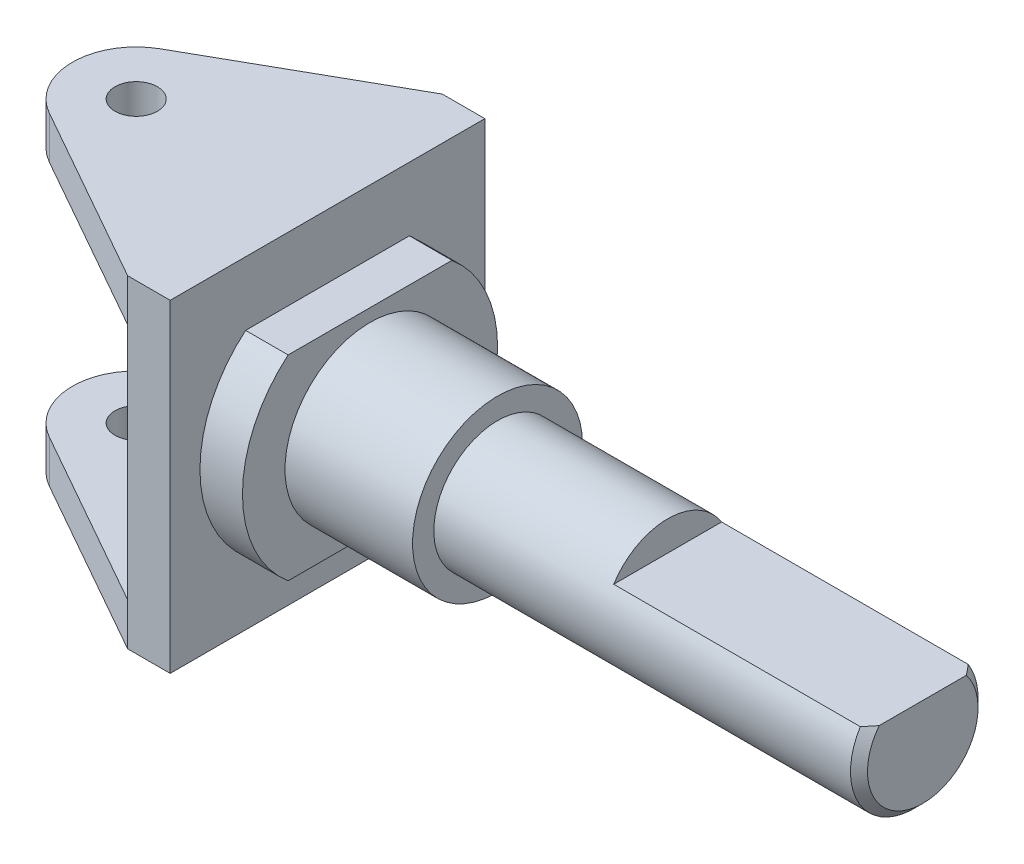
ISO-10303-21;
HEADER;
FILE_DESCRIPTION(('STEP AP214'),'2;1');
FILE_NAME('part.step','',(''),(''),'','','');
FILE_SCHEMA(('AUTOMOTIVE_DESIGN { 1 0 10303 214 1 1 1 1 }'));
ENDSEC;
DATA;
#1=APPLICATION_CONTEXT('core data for automotive mechanical design processes');
#2=APPLICATION_PROTOCOL_DEFINITION('international standard','automotive_design',2000,#1);
#3=PRODUCT_CONTEXT('',#1,'mechanical');
#4=PRODUCT('Part','Part','',(#3));
#5=PRODUCT_RELATED_PRODUCT_CATEGORY('part','',(#4));
#6=PRODUCT_DEFINITION_FORMATION('','',#4);
#7=PRODUCT_DEFINITION_CONTEXT('part definition',#1,'design');
#8=PRODUCT_DEFINITION('design','',#6,#7);
#9=PRODUCT_DEFINITION_SHAPE('','',#8);
#10=(LENGTH_UNIT() NAMED_UNIT(*) SI_UNIT(.MILLI.,.METRE.));
#11=(NAMED_UNIT(*) PLANE_ANGLE_UNIT() SI_UNIT($,.RADIAN.));
#12=(NAMED_UNIT(*) SI_UNIT($,.STERADIAN.) SOLID_ANGLE_UNIT());
#13=UNCERTAINTY_MEASURE_WITH_UNIT(LENGTH_MEASURE(1.E-05),#10,'distance_accuracy_value','');
#14=(GEOMETRIC_REPRESENTATION_CONTEXT(3) GLOBAL_UNCERTAINTY_ASSIGNED_CONTEXT((#13)) GLOBAL_UNIT_ASSIGNED_CONTEXT((#10,
#11,#12)) REPRESENTATION_CONTEXT('',''));
#15=CARTESIAN_POINT('',(0.,0.,0.));
#16=DIRECTION('',(0.,0.,1.));
#17=DIRECTION('',(1.,0.,0.));
#18=AXIS2_PLACEMENT_3D('',#15,#16,#17);
#19=CARTESIAN_POINT('',(-10.,38.,-74.));
#20=DIRECTION('',(-1.,0.,0.));
#21=DIRECTION('',(0.,0.,1.));
#22=AXIS2_PLACEMENT_3D('',#19,#20,#21);
#23=PLANE('',#22);
#24=DIRECTION('',(0.,-1.,0.));
#25=VECTOR('',#24,1.);
#26=CARTESIAN_POINT('',(-10.,38.,-74.));
#27=LINE('',#26,#25);
#28=CARTESIAN_POINT('',(-10.,28.,-74.));
#29=VERTEX_POINT('',#28);
#30=CARTESIAN_POINT('',(-10.,-28.,-74.));
#31=VERTEX_POINT('',#30);
#32=EDGE_CURVE('E300',#29,#31,#27,.T.);
#33=ORIENTED_EDGE('',*,*,#32,.T.);
#34=DIRECTION('',(0.,0.,1.));
#35=VECTOR('',#34,1.);
#36=CARTESIAN_POINT('',(-10.,-28.,0.));
#37=LINE('',#36,#35);
#38=CARTESIAN_POINT('',(-10.,-28.,0.));
#39=VERTEX_POINT('',#38);
#40=EDGE_CURVE('E241',#31,#39,#37,.T.);
#41=ORIENTED_EDGE('',*,*,#40,.T.);
#42=DIRECTION('',(0.,-1.,0.));
#43=VECTOR('',#42,1.);
#44=CARTESIAN_POINT('',(-10.,38.,0.));
#45=LINE('',#44,#43);
#46=CARTESIAN_POINT('',(-10.,28.,0.));
#47=VERTEX_POINT('',#46);
#48=EDGE_CURVE('E292',#47,#39,#45,.T.);
#49=ORIENTED_EDGE('',*,*,#48,.F.);
#50=DIRECTION('',(0.,0.,-1.));
#51=VECTOR('',#50,1.);
#52=CARTESIAN_POINT('',(-10.,28.,-74.));
#53=LINE('',#52,#51);
#54=EDGE_CURVE('E274',#47,#29,#53,.T.);
#55=ORIENTED_EDGE('',*,*,#54,.T.);
#56=EDGE_LOOP('',(#33,#41,#49,#55));
#57=FACE_BOUND('',#56,.T.);
#58=ADVANCED_FACE('F50',(#57),#23,.T.);
#59=CARTESIAN_POINT('',(0.,38.,-74.));
#60=DIRECTION('',(0.,1.,0.));
#61=DIRECTION('',(0.,0.,1.));
#62=AXIS2_PLACEMENT_3D('',#59,#60,#61);
#63=PLANE('',#62);
#64=CARTESIAN_POINT('',(-45.,38.,-37.));
#65=DIRECTION('',(0.,1.,0.));
#66=DIRECTION('',(0.,0.,1.));
#67=AXIS2_PLACEMENT_3D('',#64,#65,#66);
#68=CIRCLE('',#67,5.);
#69=CARTESIAN_POINT('',(-45.,38.,-32.));
#70=VERTEX_POINT('',#69);
#71=EDGE_CURVE('E233',#70,#70,#68,.T.);
#72=ORIENTED_EDGE('',*,*,#71,.F.);
#73=EDGE_LOOP('',(#72));
#74=FACE_BOUND('',#73,.T.);
#75=DIRECTION('',(-1.,0.,0.));
#76=VECTOR('',#75,1.);
#77=CARTESIAN_POINT('',(0.,38.,0.));
#78=LINE('',#77,#76);
#79=CARTESIAN_POINT('',(0.,38.,0.));
#80=VERTEX_POINT('',#79);
#81=CARTESIAN_POINT('',(-10.,38.,0.));
#82=VERTEX_POINT('',#81);
#83=EDGE_CURVE('E316',#80,#82,#78,.T.);
#84=ORIENTED_EDGE('',*,*,#83,.F.);
#85=DIRECTION('',(0.,0.,1.));
#86=VECTOR('',#85,1.);
#87=CARTESIAN_POINT('',(0.,38.,-74.));
#88=LINE('',#87,#86);
#89=CARTESIAN_POINT('',(0.,38.,-74.));
#90=VERTEX_POINT('',#89);
#91=EDGE_CURVE('E193',#90,#80,#88,.T.);
#92=ORIENTED_EDGE('',*,*,#91,.F.);
#93=DIRECTION('',(-1.,0.,0.));
#94=VECTOR('',#93,1.);
#95=CARTESIAN_POINT('',(0.,38.,-74.));
#96=LINE('',#95,#94);
#97=CARTESIAN_POINT('',(-10.,38.,-74.));
#98=VERTEX_POINT('',#97);
#99=EDGE_CURVE('E305',#90,#98,#96,.T.);
#100=ORIENTED_EDGE('',*,*,#99,.T.);
#101=DIRECTION('',(-0.870675826256482,0.,0.491857302042567));
#102=VECTOR('',#101,1.);
#103=CARTESIAN_POINT('',(-52.3778595306385,38.,-50.0601373938472));
#104=LINE('',#103,#102);
#105=CARTESIAN_POINT('',(-52.3778595306385,38.,-50.0601373938472));
#106=VERTEX_POINT('',#105);
#107=EDGE_CURVE('E275',#98,#106,#104,.T.);
#108=ORIENTED_EDGE('',*,*,#107,.T.);
#109=CARTESIAN_POINT('',(-45.,38.,-37.));
#110=DIRECTION('',(0.,1.,0.));
#111=DIRECTION('',(0.,0.,1.));
#112=AXIS2_PLACEMENT_3D('',#109,#110,#111);
#113=CIRCLE('',#112,15.);
#114=CARTESIAN_POINT('',(-52.3778595306385,38.,-23.9398626061528));
#115=VERTEX_POINT('',#114);
#116=EDGE_CURVE('E261',#106,#115,#113,.T.);
#117=ORIENTED_EDGE('',*,*,#116,.T.);
#118=DIRECTION('',(0.870675826256482,0.,0.491857302042567));
#119=VECTOR('',#118,1.);
#120=CARTESIAN_POINT('',(-52.3778595306385,38.,-23.9398626061528));
#121=LINE('',#120,#119);
#122=EDGE_CURVE('E284',#115,#82,#121,.T.);
#123=ORIENTED_EDGE('',*,*,#122,.T.);
#124=EDGE_LOOP('',(#84,#92,#100,#108,#117,#123));
#125=FACE_BOUND('',#124,.T.);
#126=ADVANCED_FACE('F419',(#74,#125),#63,.T.);
#127=CARTESIAN_POINT('',(0.,-38.,-74.));
#128=DIRECTION('',(1.,0.,0.));
#129=DIRECTION('',(0.,0.,-1.));
#130=AXIS2_PLACEMENT_3D('',#127,#128,#129);
#131=PLANE('',#130);
#132=CARTESIAN_POINT('',(0.,0.,-37.));
#133=DIRECTION('',(1.,0.,0.));
#134=DIRECTION('',(0.,0.,-1.));
#135=AXIS2_PLACEMENT_3D('',#132,#133,#134);
#136=CIRCLE('',#135,30.);
#137=CARTESIAN_POINT('',(0.,-23.,-56.2613602842582));
#138=VERTEX_POINT('',#137);
#139=CARTESIAN_POINT('',(0.,23.,-56.2613602842582));
#140=VERTEX_POINT('',#139);
#141=EDGE_CURVE('E194',#138,#140,#136,.T.);
#142=ORIENTED_EDGE('',*,*,#141,.F.);
#143=DIRECTION('',(0.,0.,-1.));
#144=VECTOR('',#143,1.);
#145=CARTESIAN_POINT('',(0.,-23.,-17.7386397157418));
#146=LINE('',#145,#144);
#147=CARTESIAN_POINT('',(0.,-23.,-17.7386397157418));
#148=VERTEX_POINT('',#147);
#149=EDGE_CURVE('E200',#148,#138,#146,.T.);
#150=ORIENTED_EDGE('',*,*,#149,.F.);
#151=CARTESIAN_POINT('',(0.,0.,-37.));
#152=DIRECTION('',(1.,0.,0.));
#153=DIRECTION('',(0.,0.,-1.));
#154=AXIS2_PLACEMENT_3D('',#151,#152,#153);
#155=CIRCLE('',#154,30.);
#156=CARTESIAN_POINT('',(0.,23.,-17.7386397157418));
#157=VERTEX_POINT('',#156);
#158=EDGE_CURVE('E211',#157,#148,#155,.T.);
#159=ORIENTED_EDGE('',*,*,#158,.F.);
#160=DIRECTION('',(0.,0.,1.));
#161=VECTOR('',#160,1.);
#162=CARTESIAN_POINT('',(0.,23.,-17.7386397157418));
#163=LINE('',#162,#161);
#164=EDGE_CURVE('E208',#140,#157,#163,.T.);
#165=ORIENTED_EDGE('',*,*,#164,.F.);
#166=EDGE_LOOP('',(#142,#150,#159,#165));
#167=FACE_BOUND('',#166,.T.);
#168=DIRECTION('',(0.,1.,0.));
#169=VECTOR('',#168,1.);
#170=CARTESIAN_POINT('',(0.,-38.,0.));
#171=LINE('',#170,#169);
#172=CARTESIAN_POINT('',(0.,-38.,0.));
#173=VERTEX_POINT('',#172);
#174=EDGE_CURVE('E311',#173,#80,#171,.T.);
#175=ORIENTED_EDGE('',*,*,#174,.F.);
#176=DIRECTION('',(0.,0.,1.));
#177=VECTOR('',#176,1.);
#178=CARTESIAN_POINT('',(0.,-38.,-74.));
#179=LINE('',#178,#177);
#180=CARTESIAN_POINT('',(0.,-38.,-74.));
#181=VERTEX_POINT('',#180);
#182=EDGE_CURVE('E308',#181,#173,#179,.T.);
#183=ORIENTED_EDGE('',*,*,#182,.F.);
#184=DIRECTION('',(0.,1.,0.));
#185=VECTOR('',#184,1.);
#186=CARTESIAN_POINT('',(0.,-38.,-74.));
#187=LINE('',#186,#185);
#188=EDGE_CURVE('E296',#181,#90,#187,.T.);
#189=ORIENTED_EDGE('',*,*,#188,.T.);
#190=ORIENTED_EDGE('',*,*,#91,.T.);
#191=EDGE_LOOP('',(#175,#183,#189,#190));
#192=FACE_BOUND('',#191,.T.);
#193=ADVANCED_FACE('F421',(#167,#192),#131,.T.);
#194=CARTESIAN_POINT('',(-10.,-38.,-74.));
#195=DIRECTION('',(0.,-1.,0.));
#196=DIRECTION('',(0.,0.,-1.));
#197=AXIS2_PLACEMENT_3D('',#194,#195,#196);
#198=PLANE('',#197);
#199=CARTESIAN_POINT('',(-45.,-38.,-37.));
#200=DIRECTION('',(0.,-1.,0.));
#201=DIRECTION('',(0.,0.,-1.));
#202=AXIS2_PLACEMENT_3D('',#199,#200,#201);
#203=CIRCLE('',#202,5.);
#204=CARTESIAN_POINT('',(-45.,-38.,-42.));
#205=VERTEX_POINT('',#204);
#206=EDGE_CURVE('E230',#205,#205,#203,.T.);
#207=ORIENTED_EDGE('',*,*,#206,.F.);
#208=EDGE_LOOP('',(#207));
#209=FACE_BOUND('',#208,.T.);
#210=DIRECTION('',(1.,0.,0.));
#211=VECTOR('',#210,1.);
#212=CARTESIAN_POINT('',(-10.,-38.,0.));
#213=LINE('',#212,#211);
#214=CARTESIAN_POINT('',(-10.,-38.,0.));
#215=VERTEX_POINT('',#214);
#216=EDGE_CURVE('E309',#215,#173,#213,.T.);
#217=ORIENTED_EDGE('',*,*,#216,.F.);
#218=DIRECTION('',(-0.870675826256482,0.,-0.491857302042567));
#219=VECTOR('',#218,1.);
#220=CARTESIAN_POINT('',(-52.3778595306385,-38.,-23.9398626061528));
#221=LINE('',#220,#219);
#222=CARTESIAN_POINT('',(-52.3778595306385,-38.,-23.9398626061528));
#223=VERTEX_POINT('',#222);
#224=EDGE_CURVE('E245',#215,#223,#221,.T.);
#225=ORIENTED_EDGE('',*,*,#224,.T.);
#226=CARTESIAN_POINT('',(-45.,-38.,-37.));
#227=DIRECTION('',(0.,-1.,0.));
#228=DIRECTION('',(0.,0.,-1.));
#229=AXIS2_PLACEMENT_3D('',#226,#227,#228);
#230=CIRCLE('',#229,15.);
#231=CARTESIAN_POINT('',(-52.3778595306385,-38.,-50.0601373938472));
#232=VERTEX_POINT('',#231);
#233=EDGE_CURVE('E240',#223,#232,#230,.T.);
#234=ORIENTED_EDGE('',*,*,#233,.T.);
#235=DIRECTION('',(0.870675826256482,0.,-0.491857302042567));
#236=VECTOR('',#235,1.);
#237=CARTESIAN_POINT('',(-10.,-38.,-74.));
#238=LINE('',#237,#236);
#239=CARTESIAN_POINT('',(-10.,-38.,-74.));
#240=VERTEX_POINT('',#239);
#241=EDGE_CURVE('E255',#232,#240,#238,.T.);
#242=ORIENTED_EDGE('',*,*,#241,.T.);
#243=DIRECTION('',(1.,0.,0.));
#244=VECTOR('',#243,1.);
#245=CARTESIAN_POINT('',(-10.,-38.,-74.));
#246=LINE('',#245,#244);
#247=EDGE_CURVE('E297',#240,#181,#246,.T.);
#248=ORIENTED_EDGE('',*,*,#247,.T.);
#249=ORIENTED_EDGE('',*,*,#182,.T.);
#250=EDGE_LOOP('',(#217,#225,#234,#242,#248,#249));
#251=FACE_BOUND('',#250,.T.);
#252=ADVANCED_FACE('F412',(#209,#251),#198,.T.);
#253=CARTESIAN_POINT('',(0.,0.,-74.));
#254=DIRECTION('',(0.,0.,1.));
#255=DIRECTION('',(1.,0.,0.));
#256=AXIS2_PLACEMENT_3D('',#253,#254,#255);
#257=PLANE('',#256);
#258=EDGE_CURVE('E291',#98,#29,#27,.T.);
#259=ORIENTED_EDGE('',*,*,#258,.F.);
#260=ORIENTED_EDGE('',*,*,#99,.F.);
#261=ORIENTED_EDGE('',*,*,#188,.F.);
#262=ORIENTED_EDGE('',*,*,#247,.F.);
#263=DIRECTION('',(0.,-1.,0.));
#264=VECTOR('',#263,1.);
#265=CARTESIAN_POINT('',(-10.,-28.,-74.));
#266=LINE('',#265,#264);
#267=EDGE_CURVE('E264',#31,#240,#266,.T.);
#268=ORIENTED_EDGE('',*,*,#267,.F.);
#269=ORIENTED_EDGE('',*,*,#32,.F.);
#270=EDGE_LOOP('',(#259,#260,#261,#262,#268,#269));
#271=FACE_BOUND('',#270,.T.);
#272=ADVANCED_FACE('F411',(#271),#257,.F.);
#273=CARTESIAN_POINT('',(0.,0.,0.));
#274=DIRECTION('',(0.,0.,1.));
#275=DIRECTION('',(1.,0.,0.));
#276=AXIS2_PLACEMENT_3D('',#273,#274,#275);
#277=PLANE('',#276);
#278=EDGE_CURVE('E307',#82,#47,#45,.T.);
#279=ORIENTED_EDGE('',*,*,#278,.T.);
#280=ORIENTED_EDGE('',*,*,#48,.T.);
#281=DIRECTION('',(0.,-1.,0.));
#282=VECTOR('',#281,1.);
#283=CARTESIAN_POINT('',(-10.,-28.,0.));
#284=LINE('',#283,#282);
#285=EDGE_CURVE('E265',#39,#215,#284,.T.);
#286=ORIENTED_EDGE('',*,*,#285,.T.);
#287=ORIENTED_EDGE('',*,*,#216,.T.);
#288=ORIENTED_EDGE('',*,*,#174,.T.);
#289=ORIENTED_EDGE('',*,*,#83,.T.);
#290=EDGE_LOOP('',(#279,#280,#286,#287,#288,#289));
#291=FACE_BOUND('',#290,.T.);
#292=ADVANCED_FACE('F406',(#291),#277,.T.);
#293=CARTESIAN_POINT('',(-45.,28.,-37.));
#294=DIRECTION('',(0.,1.,0.));
#295=DIRECTION('',(0.,0.,1.));
#296=AXIS2_PLACEMENT_3D('',#293,#294,#295);
#297=CYLINDRICAL_SURFACE('',#296,15.);
#298=ORIENTED_EDGE('',*,*,#116,.F.);
#299=DIRECTION('',(0.,1.,0.));
#300=VECTOR('',#299,1.);
#301=CARTESIAN_POINT('',(-52.3778595306385,28.,-50.0601373938472));
#302=LINE('',#301,#300);
#303=CARTESIAN_POINT('',(-52.3778595306385,28.,-50.0601373938472));
#304=VERTEX_POINT('',#303);
#305=EDGE_CURVE('E288',#304,#106,#302,.T.);
#306=ORIENTED_EDGE('',*,*,#305,.F.);
#307=CARTESIAN_POINT('',(-45.,28.,-37.));
#308=DIRECTION('',(0.,1.,0.));
#309=DIRECTION('',(0.,0.,1.));
#310=AXIS2_PLACEMENT_3D('',#307,#308,#309);
#311=CIRCLE('',#310,15.);
#312=CARTESIAN_POINT('',(-52.3778595306385,28.,-23.9398626061528));
#313=VERTEX_POINT('',#312);
#314=EDGE_CURVE('E268',#304,#313,#311,.T.);
#315=ORIENTED_EDGE('',*,*,#314,.T.);
#316=DIRECTION('',(0.,1.,0.));
#317=VECTOR('',#316,1.);
#318=CARTESIAN_POINT('',(-52.3778595306385,28.,-23.9398626061528));
#319=LINE('',#318,#317);
#320=EDGE_CURVE('E282',#313,#115,#319,.T.);
#321=ORIENTED_EDGE('',*,*,#320,.T.);
#322=EDGE_LOOP('',(#298,#306,#315,#321));
#323=FACE_BOUND('',#322,.T.);
#324=ADVANCED_FACE('F401',(#323),#297,.T.);
#325=CARTESIAN_POINT('',(-52.3778595306385,28.,-50.0601373938472));
#326=DIRECTION('',(-0.491857302042566,0.,-0.870675826256482));
#327=DIRECTION('',(-0.870675826256482,0.,0.491857302042566));
#328=AXIS2_PLACEMENT_3D('',#325,#326,#327);
#329=PLANE('',#328);
#330=ORIENTED_EDGE('',*,*,#107,.F.);
#331=ORIENTED_EDGE('',*,*,#258,.T.);
#332=DIRECTION('',(-0.870675826256482,0.,0.491857302042567));
#333=VECTOR('',#332,1.);
#334=CARTESIAN_POINT('',(-52.3778595306385,28.,-50.0601373938472));
#335=LINE('',#334,#333);
#336=EDGE_CURVE('E279',#29,#304,#335,.T.);
#337=ORIENTED_EDGE('',*,*,#336,.T.);
#338=ORIENTED_EDGE('',*,*,#305,.T.);
#339=EDGE_LOOP('',(#330,#331,#337,#338));
#340=FACE_BOUND('',#339,.T.);
#341=ADVANCED_FACE('F397',(#340),#329,.T.);
#342=CARTESIAN_POINT('',(-52.3778595306385,28.,-23.9398626061528));
#343=DIRECTION('',(-0.491857302042567,0.,0.870675826256482));
#344=DIRECTION('',(0.870675826256482,0.,0.491857302042567));
#345=AXIS2_PLACEMENT_3D('',#342,#343,#344);
#346=PLANE('',#345);
#347=ORIENTED_EDGE('',*,*,#122,.F.);
#348=ORIENTED_EDGE('',*,*,#320,.F.);
#349=DIRECTION('',(0.870675826256482,0.,0.491857302042567));
#350=VECTOR('',#349,1.);
#351=CARTESIAN_POINT('',(-52.3778595306385,28.,-23.9398626061528));
#352=LINE('',#351,#350);
#353=EDGE_CURVE('E271',#313,#47,#352,.T.);
#354=ORIENTED_EDGE('',*,*,#353,.T.);
#355=ORIENTED_EDGE('',*,*,#278,.F.);
#356=EDGE_LOOP('',(#347,#348,#354,#355));
#357=FACE_BOUND('',#356,.T.);
#358=ADVANCED_FACE('F400',(#357),#346,.T.);
#359=CARTESIAN_POINT('',(-45.,28.,-37.));
#360=DIRECTION('',(0.,1.,0.));
#361=DIRECTION('',(0.,0.,1.));
#362=AXIS2_PLACEMENT_3D('',#359,#360,#361);
#363=PLANE('',#362);
#364=CARTESIAN_POINT('',(-45.,28.,-37.));
#365=DIRECTION('',(0.,1.,0.));
#366=DIRECTION('',(0.,0.,1.));
#367=AXIS2_PLACEMENT_3D('',#364,#365,#366);
#368=CIRCLE('',#367,5.);
#369=CARTESIAN_POINT('',(-45.,28.,-32.));
#370=VERTEX_POINT('',#369);
#371=EDGE_CURVE('E234',#370,#370,#368,.T.);
#372=ORIENTED_EDGE('',*,*,#371,.T.);
#373=EDGE_LOOP('',(#372));
#374=FACE_BOUND('',#373,.T.);
#375=ORIENTED_EDGE('',*,*,#314,.F.);
#376=ORIENTED_EDGE('',*,*,#336,.F.);
#377=ORIENTED_EDGE('',*,*,#54,.F.);
#378=ORIENTED_EDGE('',*,*,#353,.F.);
#379=EDGE_LOOP('',(#375,#376,#377,#378));
#380=FACE_BOUND('',#379,.T.);
#381=ADVANCED_FACE('F394',(#374,#380),#363,.F.);
#382=CARTESIAN_POINT('',(-45.,-28.,-37.));
#383=DIRECTION('',(0.,-1.,0.));
#384=DIRECTION('',(0.,0.,-1.));
#385=AXIS2_PLACEMENT_3D('',#382,#383,#384);
#386=CYLINDRICAL_SURFACE('',#385,15.);
#387=ORIENTED_EDGE('',*,*,#233,.F.);
#388=DIRECTION('',(0.,-1.,0.));
#389=VECTOR('',#388,1.);
#390=CARTESIAN_POINT('',(-52.3778595306385,-28.,-23.9398626061528));
#391=LINE('',#390,#389);
#392=CARTESIAN_POINT('',(-52.3778595306385,-28.,-23.9398626061528));
#393=VERTEX_POINT('',#392);
#394=EDGE_CURVE('E259',#393,#223,#391,.T.);
#395=ORIENTED_EDGE('',*,*,#394,.F.);
#396=CARTESIAN_POINT('',(-45.,-28.,-37.));
#397=DIRECTION('',(0.,-1.,0.));
#398=DIRECTION('',(0.,0.,-1.));
#399=AXIS2_PLACEMENT_3D('',#396,#397,#398);
#400=CIRCLE('',#399,15.);
#401=CARTESIAN_POINT('',(-52.3778595306385,-28.,-50.0601373938472));
#402=VERTEX_POINT('',#401);
#403=EDGE_CURVE('E236',#393,#402,#400,.T.);
#404=ORIENTED_EDGE('',*,*,#403,.T.);
#405=DIRECTION('',(0.,-1.,0.));
#406=VECTOR('',#405,1.);
#407=CARTESIAN_POINT('',(-52.3778595306385,-28.,-50.0601373938472));
#408=LINE('',#407,#406);
#409=EDGE_CURVE('E253',#402,#232,#408,.T.);
#410=ORIENTED_EDGE('',*,*,#409,.T.);
#411=EDGE_LOOP('',(#387,#395,#404,#410));
#412=FACE_BOUND('',#411,.T.);
#413=ADVANCED_FACE('F390',(#412),#386,.T.);
#414=CARTESIAN_POINT('',(-52.3778595306385,-28.,-23.9398626061528));
#415=DIRECTION('',(-0.491857302042567,0.,0.870675826256482));
#416=DIRECTION('',(0.870675826256482,0.,0.491857302042567));
#417=AXIS2_PLACEMENT_3D('',#414,#415,#416);
#418=PLANE('',#417);
#419=ORIENTED_EDGE('',*,*,#224,.F.);
#420=ORIENTED_EDGE('',*,*,#285,.F.);
#421=DIRECTION('',(-0.870675826256482,0.,-0.491857302042567));
#422=VECTOR('',#421,1.);
#423=CARTESIAN_POINT('',(-52.3778595306385,-28.,-23.9398626061528));
#424=LINE('',#423,#422);
#425=EDGE_CURVE('E250',#39,#393,#424,.T.);
#426=ORIENTED_EDGE('',*,*,#425,.T.);
#427=ORIENTED_EDGE('',*,*,#394,.T.);
#428=EDGE_LOOP('',(#419,#420,#426,#427));
#429=FACE_BOUND('',#428,.T.);
#430=ADVANCED_FACE('F383',(#429),#418,.T.);
#431=CARTESIAN_POINT('',(-10.,-28.,-74.));
#432=DIRECTION('',(-0.491857302042566,0.,-0.870675826256482));
#433=DIRECTION('',(-0.870675826256482,0.,0.491857302042566));
#434=AXIS2_PLACEMENT_3D('',#431,#432,#433);
#435=PLANE('',#434);
#436=ORIENTED_EDGE('',*,*,#241,.F.);
#437=ORIENTED_EDGE('',*,*,#409,.F.);
#438=DIRECTION('',(0.870675826256482,0.,-0.491857302042567));
#439=VECTOR('',#438,1.);
#440=CARTESIAN_POINT('',(-10.,-28.,-74.));
#441=LINE('',#440,#439);
#442=EDGE_CURVE('E242',#402,#31,#441,.T.);
#443=ORIENTED_EDGE('',*,*,#442,.T.);
#444=ORIENTED_EDGE('',*,*,#267,.T.);
#445=EDGE_LOOP('',(#436,#437,#443,#444));
#446=FACE_BOUND('',#445,.T.);
#447=ADVANCED_FACE('F385',(#446),#435,.T.);
#448=CARTESIAN_POINT('',(-45.,-28.,-37.));
#449=DIRECTION('',(0.,-1.,0.));
#450=DIRECTION('',(0.,0.,-1.));
#451=AXIS2_PLACEMENT_3D('',#448,#449,#450);
#452=PLANE('',#451);
#453=CARTESIAN_POINT('',(-45.,-28.,-37.));
#454=DIRECTION('',(0.,-1.,0.));
#455=DIRECTION('',(0.,0.,-1.));
#456=AXIS2_PLACEMENT_3D('',#453,#454,#455);
#457=CIRCLE('',#456,5.);
#458=CARTESIAN_POINT('',(-45.,-28.,-42.));
#459=VERTEX_POINT('',#458);
#460=EDGE_CURVE('E226',#459,#459,#457,.T.);
#461=ORIENTED_EDGE('',*,*,#460,.T.);
#462=EDGE_LOOP('',(#461));
#463=FACE_BOUND('',#462,.T.);
#464=ORIENTED_EDGE('',*,*,#403,.F.);
#465=ORIENTED_EDGE('',*,*,#425,.F.);
#466=ORIENTED_EDGE('',*,*,#40,.F.);
#467=ORIENTED_EDGE('',*,*,#442,.F.);
#468=EDGE_LOOP('',(#464,#465,#466,#467));
#469=FACE_BOUND('',#468,.T.);
#470=ADVANCED_FACE('F377',(#463,#469),#452,.F.);
#471=CARTESIAN_POINT('',(-45.,62.,-37.));
#472=DIRECTION('',(0.,-1.,0.));
#473=DIRECTION('',(0.,0.,-1.));
#474=AXIS2_PLACEMENT_3D('',#471,#472,#473);
#475=CYLINDRICAL_SURFACE('',#474,5.);
#476=ORIENTED_EDGE('',*,*,#206,.T.);
#477=EDGE_LOOP('',(#476));
#478=FACE_BOUND('',#477,.T.);
#479=ORIENTED_EDGE('',*,*,#460,.F.);
#480=EDGE_LOOP('',(#479));
#481=FACE_BOUND('',#480,.T.);
#482=ADVANCED_FACE('F380',(#478,#481),#475,.F.);
#483=ORIENTED_EDGE('',*,*,#71,.T.);
#484=EDGE_LOOP('',(#483));
#485=FACE_BOUND('',#484,.T.);
#486=ORIENTED_EDGE('',*,*,#371,.F.);
#487=EDGE_LOOP('',(#486));
#488=FACE_BOUND('',#487,.T.);
#489=ADVANCED_FACE('F373',(#485,#488),#475,.F.);
#490=CARTESIAN_POINT('',(10.,0.,-37.));
#491=DIRECTION('',(-1.,0.,0.));
#492=DIRECTION('',(0.,0.,1.));
#493=AXIS2_PLACEMENT_3D('',#490,#491,#492);
#494=CYLINDRICAL_SURFACE('',#493,30.);
#495=ORIENTED_EDGE('',*,*,#141,.T.);
#496=DIRECTION('',(-1.,0.,0.));
#497=VECTOR('',#496,1.);
#498=CARTESIAN_POINT('',(10.,23.,-56.2613602842582));
#499=LINE('',#498,#497);
#500=CARTESIAN_POINT('',(10.,23.,-56.2613602842582));
#501=VERTEX_POINT('',#500);
#502=EDGE_CURVE('E221',#501,#140,#499,.T.);
#503=ORIENTED_EDGE('',*,*,#502,.F.);
#504=CARTESIAN_POINT('',(10.,0.,-37.));
#505=DIRECTION('',(1.,0.,0.));
#506=DIRECTION('',(0.,0.,-1.));
#507=AXIS2_PLACEMENT_3D('',#504,#505,#506);
#508=CIRCLE('',#507,30.);
#509=CARTESIAN_POINT('',(10.,-23.,-56.2613602842582));
#510=VERTEX_POINT('',#509);
#511=EDGE_CURVE('E192',#510,#501,#508,.T.);
#512=ORIENTED_EDGE('',*,*,#511,.F.);
#513=DIRECTION('',(-1.,0.,0.));
#514=VECTOR('',#513,1.);
#515=CARTESIAN_POINT('',(10.,-23.,-56.2613602842582));
#516=LINE('',#515,#514);
#517=EDGE_CURVE('E202',#510,#138,#516,.T.);
#518=ORIENTED_EDGE('',*,*,#517,.T.);
#519=EDGE_LOOP('',(#495,#503,#512,#518));
#520=FACE_BOUND('',#519,.T.);
#521=ADVANCED_FACE('F369',(#520),#494,.T.);
#522=CARTESIAN_POINT('',(10.,23.,-17.7386397157418));
#523=DIRECTION('',(0.,-1.,0.));
#524=DIRECTION('',(0.,0.,-1.));
#525=AXIS2_PLACEMENT_3D('',#522,#523,#524);
#526=PLANE('',#525);
#527=ORIENTED_EDGE('',*,*,#164,.T.);
#528=DIRECTION('',(-1.,0.,0.));
#529=VECTOR('',#528,1.);
#530=CARTESIAN_POINT('',(10.,23.,-17.7386397157418));
#531=LINE('',#530,#529);
#532=CARTESIAN_POINT('',(10.,23.,-17.7386397157418));
#533=VERTEX_POINT('',#532);
#534=EDGE_CURVE('E222',#533,#157,#531,.T.);
#535=ORIENTED_EDGE('',*,*,#534,.F.);
#536=DIRECTION('',(0.,0.,1.));
#537=VECTOR('',#536,1.);
#538=CARTESIAN_POINT('',(10.,23.,-17.7386397157418));
#539=LINE('',#538,#537);
#540=EDGE_CURVE('E196',#501,#533,#539,.T.);
#541=ORIENTED_EDGE('',*,*,#540,.F.);
#542=ORIENTED_EDGE('',*,*,#502,.T.);
#543=EDGE_LOOP('',(#527,#535,#541,#542));
#544=FACE_BOUND('',#543,.T.);
#545=ADVANCED_FACE('F364',(#544),#526,.F.);
#546=CARTESIAN_POINT('',(10.,0.,-37.));
#547=DIRECTION('',(-1.,0.,0.));
#548=DIRECTION('',(0.,0.,1.));
#549=AXIS2_PLACEMENT_3D('',#546,#547,#548);
#550=CYLINDRICAL_SURFACE('',#549,30.);
#551=ORIENTED_EDGE('',*,*,#158,.T.);
#552=DIRECTION('',(-1.,0.,0.));
#553=VECTOR('',#552,1.);
#554=CARTESIAN_POINT('',(10.,-23.,-17.7386397157418));
#555=LINE('',#554,#553);
#556=CARTESIAN_POINT('',(10.,-23.,-17.7386397157418));
#557=VERTEX_POINT('',#556);
#558=EDGE_CURVE('E217',#557,#148,#555,.T.);
#559=ORIENTED_EDGE('',*,*,#558,.F.);
#560=CARTESIAN_POINT('',(10.,0.,-37.));
#561=DIRECTION('',(1.,0.,0.));
#562=DIRECTION('',(0.,0.,-1.));
#563=AXIS2_PLACEMENT_3D('',#560,#561,#562);
#564=CIRCLE('',#563,30.);
#565=EDGE_CURVE('E203',#533,#557,#564,.T.);
#566=ORIENTED_EDGE('',*,*,#565,.F.);
#567=ORIENTED_EDGE('',*,*,#534,.T.);
#568=EDGE_LOOP('',(#551,#559,#566,#567));
#569=FACE_BOUND('',#568,.T.);
#570=ADVANCED_FACE('F363',(#569),#550,.T.);
#571=CARTESIAN_POINT('',(10.,-23.,-17.7386397157418));
#572=DIRECTION('',(0.,1.,0.));
#573=DIRECTION('',(0.,0.,1.));
#574=AXIS2_PLACEMENT_3D('',#571,#572,#573);
#575=PLANE('',#574);
#576=ORIENTED_EDGE('',*,*,#149,.T.);
#577=ORIENTED_EDGE('',*,*,#517,.F.);
#578=DIRECTION('',(0.,0.,-1.));
#579=VECTOR('',#578,1.);
#580=CARTESIAN_POINT('',(10.,-23.,-17.7386397157418));
#581=LINE('',#580,#579);
#582=EDGE_CURVE('E201',#557,#510,#581,.T.);
#583=ORIENTED_EDGE('',*,*,#582,.F.);
#584=ORIENTED_EDGE('',*,*,#558,.T.);
#585=EDGE_LOOP('',(#576,#577,#583,#584));
#586=FACE_BOUND('',#585,.T.);
#587=ADVANCED_FACE('F356',(#586),#575,.F.);
#588=CARTESIAN_POINT('',(10.,0.,-37.));
#589=DIRECTION('',(1.,0.,0.));
#590=DIRECTION('',(0.,0.,-1.));
#591=AXIS2_PLACEMENT_3D('',#588,#589,#590);
#592=PLANE('',#591);
#593=CARTESIAN_POINT('',(10.,0.,-37.));
#594=DIRECTION('',(1.,0.,0.));
#595=DIRECTION('',(0.,0.,-1.));
#596=AXIS2_PLACEMENT_3D('',#593,#594,#595);
#597=CIRCLE('',#596,20.);
#598=CARTESIAN_POINT('',(10.,0.,-57.));
#599=VERTEX_POINT('',#598);
#600=EDGE_CURVE('E188',#599,#599,#597,.T.);
#601=ORIENTED_EDGE('',*,*,#600,.F.);
#602=EDGE_LOOP('',(#601));
#603=FACE_BOUND('',#602,.T.);
#604=ORIENTED_EDGE('',*,*,#511,.T.);
#605=ORIENTED_EDGE('',*,*,#540,.T.);
#606=ORIENTED_EDGE('',*,*,#565,.T.);
#607=ORIENTED_EDGE('',*,*,#582,.T.);
#608=EDGE_LOOP('',(#604,#605,#606,#607));
#609=FACE_BOUND('',#608,.T.);
#610=ADVANCED_FACE('F353',(#603,#609),#592,.T.);
#611=CARTESIAN_POINT('',(40.,0.,-37.));
#612=DIRECTION('',(-1.,0.,0.));
#613=DIRECTION('',(0.,0.,1.));
#614=AXIS2_PLACEMENT_3D('',#611,#612,#613);
#615=CYLINDRICAL_SURFACE('',#614,20.);
#616=CARTESIAN_POINT('',(40.,0.,-37.));
#617=DIRECTION('',(1.,0.,0.));
#618=DIRECTION('',(0.,0.,-1.));
#619=AXIS2_PLACEMENT_3D('',#616,#617,#618);
#620=CIRCLE('',#619,20.);
#621=CARTESIAN_POINT('',(40.,0.,-57.));
#622=VERTEX_POINT('',#621);
#623=EDGE_CURVE('E177',#622,#622,#620,.T.);
#624=ORIENTED_EDGE('',*,*,#623,.F.);
#625=EDGE_LOOP('',(#624));
#626=FACE_BOUND('',#625,.T.);
#627=ORIENTED_EDGE('',*,*,#600,.T.);
#628=EDGE_LOOP('',(#627));
#629=FACE_BOUND('',#628,.T.);
#630=ADVANCED_FACE('F349',(#626,#629),#615,.T.);
#631=CARTESIAN_POINT('',(40.,0.,-37.));
#632=DIRECTION('',(1.,0.,0.));
#633=DIRECTION('',(0.,0.,-1.));
#634=AXIS2_PLACEMENT_3D('',#631,#632,#633);
#635=PLANE('',#634);
#636=CARTESIAN_POINT('',(40.,0.,-37.));
#637=DIRECTION('',(1.,0.,0.));
#638=DIRECTION('',(0.,0.,-1.));
#639=AXIS2_PLACEMENT_3D('',#636,#637,#638);
#640=CIRCLE('',#639,15.);
#641=CARTESIAN_POINT('',(40.,0.,-52.));
#642=VERTEX_POINT('',#641);
#643=EDGE_CURVE('E184',#642,#642,#640,.T.);
#644=ORIENTED_EDGE('',*,*,#643,.F.);
#645=EDGE_LOOP('',(#644));
#646=FACE_BOUND('',#645,.T.);
#647=ORIENTED_EDGE('',*,*,#623,.T.);
#648=EDGE_LOOP('',(#647));
#649=FACE_BOUND('',#648,.T.);
#650=ADVANCED_FACE('F347',(#646,#649),#635,.T.);
#651=CARTESIAN_POINT('',(140.,0.,-37.));
#652=DIRECTION('',(-1.,0.,0.));
#653=DIRECTION('',(0.,0.,1.));
#654=AXIS2_PLACEMENT_3D('',#651,#652,#653);
#655=CYLINDRICAL_SURFACE('',#654,15.);
#656=DIRECTION('',(1.,0.,0.));
#657=VECTOR('',#656,1.);
#658=CARTESIAN_POINT('',(80.,8.,-49.6885775404495));
#659=LINE('',#658,#657);
#660=CARTESIAN_POINT('',(80.,8.,-49.6885775404495));
#661=VERTEX_POINT('',#660);
#662=CARTESIAN_POINT('',(138.,8.,-49.6885775404495));
#663=VERTEX_POINT('',#662);
#664=EDGE_CURVE('E171',#661,#663,#659,.T.);
#665=ORIENTED_EDGE('',*,*,#664,.T.);
#666=CARTESIAN_POINT('',(138.,0.,-37.));
#667=DIRECTION('',(1.,0.,0.));
#668=DIRECTION('',(0.,0.,-1.));
#669=AXIS2_PLACEMENT_3D('',#666,#667,#668);
#670=CIRCLE('',#669,15.);
#671=CARTESIAN_POINT('',(138.,8.,-24.3114224595505));
#672=VERTEX_POINT('',#671);
#673=EDGE_CURVE('E11',#663,#672,#670,.F.);
#674=ORIENTED_EDGE('',*,*,#673,.T.);
#675=DIRECTION('',(1.,0.,0.));
#676=VECTOR('',#675,1.);
#677=CARTESIAN_POINT('',(80.,8.,-24.3114224595505));
#678=LINE('',#677,#676);
#679=CARTESIAN_POINT('',(80.,8.,-24.3114224595505));
#680=VERTEX_POINT('',#679);
#681=EDGE_CURVE('E173',#680,#672,#678,.T.);
#682=ORIENTED_EDGE('',*,*,#681,.F.);
#683=CARTESIAN_POINT('',(80.,0.,-37.));
#684=DIRECTION('',(1.,0.,0.));
#685=DIRECTION('',(0.,0.,-1.));
#686=AXIS2_PLACEMENT_3D('',#683,#684,#685);
#687=CIRCLE('',#686,15.);
#688=EDGE_CURVE('E167',#661,#680,#687,.T.);
#689=ORIENTED_EDGE('',*,*,#688,.F.);
#690=EDGE_LOOP('',(#665,#674,#682,#689));
#691=FACE_BOUND('',#690,.T.);
#692=ORIENTED_EDGE('',*,*,#643,.T.);
#693=EDGE_LOOP('',(#692));
#694=FACE_BOUND('',#693,.T.);
#695=ADVANCED_FACE('F176',(#691,#694),#655,.T.);
#696=CARTESIAN_POINT('',(140.,0.,-37.));
#697=DIRECTION('',(1.,0.,0.));
#698=DIRECTION('',(0.,0.,-1.));
#699=AXIS2_PLACEMENT_3D('',#696,#697,#698);
#700=PLANE('',#699);
#701=DIRECTION('',(0.,0.,-1.));
#702=VECTOR('',#701,1.);
#703=CARTESIAN_POINT('',(140.,8.,-24.3114224595505));
#704=LINE('',#703,#702);
#705=CARTESIAN_POINT('',(140.,8.,-26.7530492340405));
#706=VERTEX_POINT('',#705);
#707=CARTESIAN_POINT('',(140.,8.,-47.2469507659595));
#708=VERTEX_POINT('',#707);
#709=EDGE_CURVE('E168',#706,#708,#704,.T.);
#710=ORIENTED_EDGE('',*,*,#709,.F.);
#711=CARTESIAN_POINT('',(140.,0.,-37.));
#712=DIRECTION('',(1.,0.,0.));
#713=DIRECTION('',(0.,0.,-1.));
#714=AXIS2_PLACEMENT_3D('',#711,#712,#713);
#715=CIRCLE('',#714,13.);
#716=EDGE_CURVE('E190',#706,#708,#715,.T.);
#717=ORIENTED_EDGE('',*,*,#716,.T.);
#718=EDGE_LOOP('',(#710,#717));
#719=FACE_BOUND('',#718,.T.);
#720=ADVANCED_FACE('F339',(#719),#700,.T.);
#721=CARTESIAN_POINT('',(80.,8.,-24.3114224595505));
#722=DIRECTION('',(0.,-1.,0.));
#723=DIRECTION('',(0.,0.,-1.));
#724=AXIS2_PLACEMENT_3D('',#721,#722,#723);
#725=PLANE('',#724);
#726=ORIENTED_EDGE('',*,*,#709,.T.);
#727=CARTESIAN_POINT('',(140.,8.,-47.2469507659595));
#728=CARTESIAN_POINT('',(139.837157689493,8.,-47.4535274279109));
#729=CARTESIAN_POINT('',(139.673183678239,8.,-47.6592075116507));
#730=CARTESIAN_POINT('',(139.343252945693,8.,-48.0689468639799));
#731=CARTESIAN_POINT('',(139.17729637193,8.,-48.2730062513122));
#732=CARTESIAN_POINT('',(138.843659587089,8.,-48.6797039469955));
#733=CARTESIAN_POINT('',(138.675979402365,8.,-48.8823422769942));
#734=CARTESIAN_POINT('',(138.339085567999,8.,-49.2863659787348));
#735=CARTESIAN_POINT('',(138.169871805975,8.,-49.4877512567981));
#736=CARTESIAN_POINT('',(138.,8.,-49.6885775404495));
#737=B_SPLINE_CURVE_WITH_KNOTS('',3,(#727,#728,#729,#730,#731,#732,#733,#734,#735,#736),
.UNSPECIFIED.,.F.,.F.,(4,2,2,2,4),(0.,0.78911950923623,1.57818065896151,2.3672297623627,
3.15633716315504),.UNSPECIFIED.);
#738=EDGE_CURVE('E60',#708,#663,#737,.T.);
#739=ORIENTED_EDGE('',*,*,#738,.T.);
#740=ORIENTED_EDGE('',*,*,#664,.F.);
#741=DIRECTION('',(0.,0.,-1.));
#742=VECTOR('',#741,1.);
#743=CARTESIAN_POINT('',(80.,8.,-24.3114224595505));
#744=LINE('',#743,#742);
#745=EDGE_CURVE('E166',#680,#661,#744,.T.);
#746=ORIENTED_EDGE('',*,*,#745,.F.);
#747=ORIENTED_EDGE('',*,*,#681,.T.);
#748=CARTESIAN_POINT('',(138.,8.,-24.3114224595505));
#749=CARTESIAN_POINT('',(138.169871805975,8.,-24.5122487432019));
#750=CARTESIAN_POINT('',(138.339085567999,8.,-24.7136340212652));
#751=CARTESIAN_POINT('',(138.675979402365,8.,-25.1176577230058));
#752=CARTESIAN_POINT('',(138.843659587089,8.,-25.3202960530045));
#753=CARTESIAN_POINT('',(139.17729637193,8.,-25.7269937486878));
#754=CARTESIAN_POINT('',(139.343252945693,8.,-25.9310531360201));
#755=CARTESIAN_POINT('',(139.673183678239,8.,-26.3407924883493));
#756=CARTESIAN_POINT('',(139.837157689493,8.,-26.5464725720891));
#757=CARTESIAN_POINT('',(140.,8.,-26.7530492340404));
#758=B_SPLINE_CURVE_WITH_KNOTS('',3,(#748,#749,#750,#751,#752,#753,#754,#755,#756,#757),
.UNSPECIFIED.,.F.,.F.,(4,2,2,2,4),(0.,0.789107400792354,1.57815650419353,2.36721765391882,
3.15633716315504),.UNSPECIFIED.);
#759=EDGE_CURVE('E324',#672,#706,#758,.T.);
#760=ORIENTED_EDGE('',*,*,#759,.T.);
#761=EDGE_LOOP('',(#726,#739,#740,#746,#747,#760));
#762=FACE_BOUND('',#761,.T.);
#763=ADVANCED_FACE('F175',(#762),#725,.F.);
#764=CARTESIAN_POINT('',(80.,0.,-37.));
#765=DIRECTION('',(1.,0.,0.));
#766=DIRECTION('',(0.,0.,-1.));
#767=AXIS2_PLACEMENT_3D('',#764,#765,#766);
#768=PLANE('',#767);
#769=ORIENTED_EDGE('',*,*,#688,.T.);
#770=ORIENTED_EDGE('',*,*,#745,.T.);
#771=EDGE_LOOP('',(#769,#770));
#772=FACE_BOUND('',#771,.T.);
#773=ADVANCED_FACE('F169',(#772),#768,.T.);
#774=CARTESIAN_POINT('',(140.,0.,-37.));
#775=DIRECTION('',(-1.,0.,0.));
#776=DIRECTION('',(0.,0.,1.));
#777=AXIS2_PLACEMENT_3D('',#774,#775,#776);
#778=CONICAL_SURFACE('',#777,13.,0.785398163397452);
#779=ORIENTED_EDGE('',*,*,#759,.F.);
#780=ORIENTED_EDGE('',*,*,#673,.F.);
#781=ORIENTED_EDGE('',*,*,#738,.F.);
#782=ORIENTED_EDGE('',*,*,#716,.F.);
#783=EDGE_LOOP('',(#779,#780,#781,#782));
#784=FACE_BOUND('',#783,.T.);
#785=ADVANCED_FACE('F49',(#784),#778,.T.);
#786=CLOSED_SHELL('',(#58,#126,#193,#252,#272,#292,#324,#341,#358,#381,#413,#430,#447,#470,#482,
#489,#521,#545,#570,#587,#610,#630,#650,#695,#720,#763,#773,#785));
#787=MANIFOLD_SOLID_BREP('B2',#786);
#788=ADVANCED_BREP_SHAPE_REPRESENTATION('',(#18,#787),#14);
#789=SHAPE_DEFINITION_REPRESENTATION(#9,#788);
ENDSEC;
END-ISO-10303-21;
